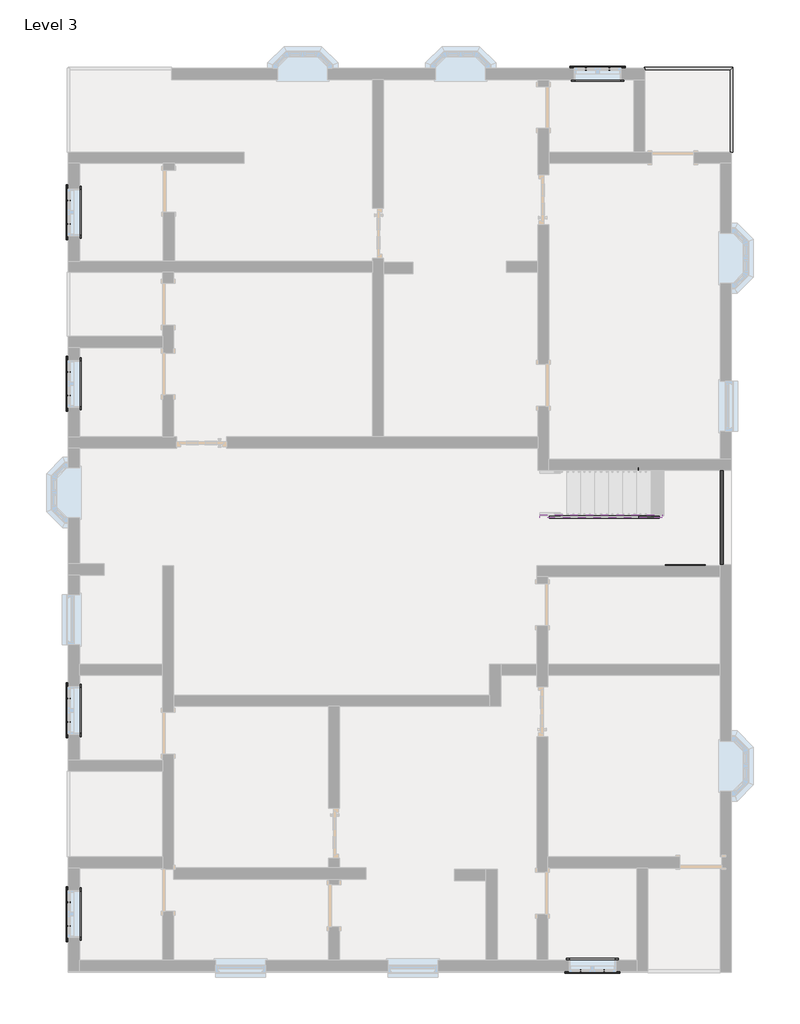
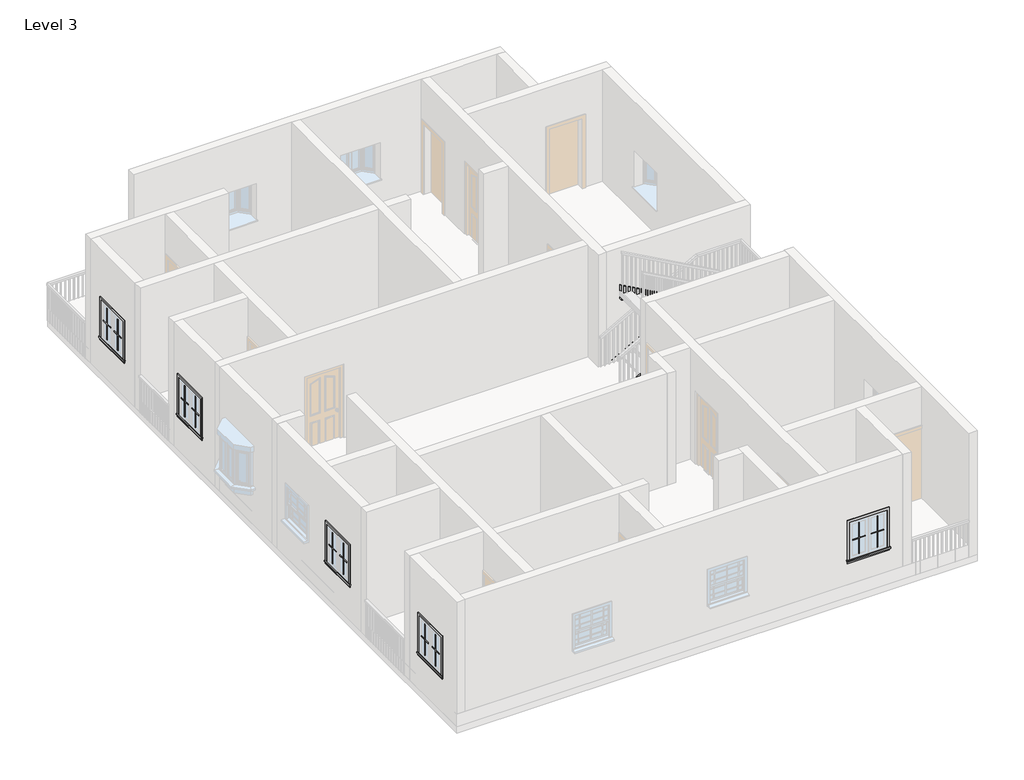
# One storey, part 4 of 4: 24 proxies, 5 members, 1 railing.
"""IFC4 building model written with IfcOpenShell, lengths in millimetres."""

from ifc_helpers import new_model, si_unit, frame, origin, place, context, project, spatial, polyline, outline, extrude, faceted_brep, transform, mapped, element, save
from components import muntin_pattern_2x2_muntin_pattern_2x2_b3fe6957, muntin_pattern_2x2_muntin_pattern_2x2_3e0ecaf2, trim_window_exterior_flat_with_sill_41619996, trim_window_interior_flat_picture_frame_51c85655

model = new_model("IFC4")

# Units and contexts
model_context = context("Model", 3, world=origin())
ifc_project = project(units=[si_unit("LENGTHUNIT", "METRE", prefix="MILLI")], contexts=[model_context])

# Site, building, storey
site = spatial("IfcSite", under=ifc_project)
building = spatial("IfcBuilding", under=site)
storey = spatial("IfcBuildingStorey", under=building, Name="Level 3", Elevation=6096.0)

# Proxies
placement = place(None, origin())
muntin_pattern_2x2_muntin_pattern_2x2_shape = muntin_pattern_2x2_muntin_pattern_2x2_b3fe6957(model_context)
element("IfcBuildingElementProxy", 1, Name="Muntin Pattern_2x2 : Muntin Pattern_2x2", ObjectType="Muntin Pattern_2x2 : Muntin Pattern_2x2", at=placement, inside=storey, context=model_context, shape_type="MappedRepresentation", body=[
    mapped(muntin_pattern_2x2_muntin_pattern_2x2_shape, transform((-7038.4808717, 5489.0318597, 7080.25), x_axis=(0.0, 1.0, 0.0), y_axis=(-1.0, 0.0, 0.0), z_axis=(0.0, 0.0, 1.0))),
])
element("IfcBuildingElementProxy", 2, Name="Muntin Pattern_2x2 : Muntin Pattern_2x2", ObjectType="Muntin Pattern_2x2 : Muntin Pattern_2x2", at=placement, inside=storey, context=model_context, shape_type="MappedRepresentation", body=[
    mapped(muntin_pattern_2x2_muntin_pattern_2x2_shape, transform((-7038.4808717, 2366.9422293, 7080.25), x_axis=(0.0, 1.0, 0.0), y_axis=(-1.0, 0.0, 0.0), z_axis=(0.0, 0.0, 1.0))),
])
element("IfcBuildingElementProxy", 3, Name="Muntin Pattern_2x2 : Muntin Pattern_2x2", ObjectType="Muntin Pattern_2x2 : Muntin Pattern_2x2", at=placement, inside=storey, context=model_context, shape_type="MappedRepresentation", body=[
    mapped(muntin_pattern_2x2_muntin_pattern_2x2_shape, transform((2376.9816283, 8312.1297293, 7080.25), x_axis=(1.0, 0.0, 0.0), y_axis=(0.0, 1.0, 0.0), z_axis=(0.0, 0.0, 1.0))),
])
element("IfcBuildingElementProxy", 4, Name="Muntin Pattern_2x2 : Muntin Pattern_2x2", ObjectType="Muntin Pattern_2x2 : Muntin Pattern_2x2", at=placement, inside=storey, context=model_context, shape_type="MappedRepresentation", body=[
    mapped(muntin_pattern_2x2_muntin_pattern_2x2_shape, transform((2710.3566283, -8102.6202707, 7080.25), x_axis=(-1.0, 0.0, 0.0), y_axis=(0.0, -1.0, 0.0), z_axis=(0.0, 0.0, 1.0))),
])
element("IfcBuildingElementProxy", 5, Name="Muntin Pattern_2x2 : Muntin Pattern_2x2", ObjectType="Muntin Pattern_2x2 : Muntin Pattern_2x2", at=placement, inside=storey, context=model_context, shape_type="MappedRepresentation", body=[
    mapped(muntin_pattern_2x2_muntin_pattern_2x2_shape, transform((-7038.4808717, -7285.0577707, 7080.25), x_axis=(0.0, 1.0, 0.0), y_axis=(-1.0, 0.0, 0.0), z_axis=(0.0, 0.0, 1.0))),
])
element("IfcBuildingElementProxy", 6, Name="Muntin Pattern_2x2 : Muntin Pattern_2x2", ObjectType="Muntin Pattern_2x2 : Muntin Pattern_2x2", at=placement, inside=storey, context=model_context, shape_type="MappedRepresentation", body=[
    mapped(muntin_pattern_2x2_muntin_pattern_2x2_shape, transform((-7038.4808717, -3576.6577707, 7080.25), x_axis=(0.0, 1.0, 0.0), y_axis=(-1.0, 0.0, 0.0), z_axis=(0.0, 0.0, 1.0))),
])
muntin_pattern_2x2_muntin_pattern_2x2_2_shape = muntin_pattern_2x2_muntin_pattern_2x2_3e0ecaf2(model_context)
element("IfcBuildingElementProxy", 7, Name="Muntin Pattern_2x2 : Muntin Pattern_2x2", ObjectType="Muntin Pattern_2x2 : Muntin Pattern_2x2", at=placement, inside=storey, context=model_context, shape_type="MappedRepresentation", body=[
    mapped(muntin_pattern_2x2_muntin_pattern_2x2_2_shape, transform((-7038.4808717, 5917.6568597, 7080.25), x_axis=(0.0, -1.0, 0.0), y_axis=(1.0, 0.0, 0.0), z_axis=(0.0, 0.0, 1.0))),
])
element("IfcBuildingElementProxy", 8, Name="Muntin Pattern_2x2 : Muntin Pattern_2x2", ObjectType="Muntin Pattern_2x2 : Muntin Pattern_2x2", at=placement, inside=storey, context=model_context, shape_type="MappedRepresentation", body=[
    mapped(muntin_pattern_2x2_muntin_pattern_2x2_2_shape, transform((-7038.4808717, 2795.5672293, 7080.25), x_axis=(0.0, -1.0, 0.0), y_axis=(1.0, 0.0, 0.0), z_axis=(0.0, 0.0, 1.0))),
])
element("IfcBuildingElementProxy", 9, Name="Muntin Pattern_2x2 : Muntin Pattern_2x2", ObjectType="Muntin Pattern_2x2 : Muntin Pattern_2x2", at=placement, inside=storey, context=model_context, shape_type="MappedRepresentation", body=[
    mapped(muntin_pattern_2x2_muntin_pattern_2x2_2_shape, transform((2805.6066283, 8312.1297293, 7080.25), x_axis=(-1.0, 0.0, 0.0), y_axis=(0.0, -1.0, 0.0), z_axis=(0.0, 0.0, 1.0))),
])
element("IfcBuildingElementProxy", 10, Name="Muntin Pattern_2x2 : Muntin Pattern_2x2", ObjectType="Muntin Pattern_2x2 : Muntin Pattern_2x2", at=placement, inside=storey, context=model_context, shape_type="MappedRepresentation", body=[
    mapped(muntin_pattern_2x2_muntin_pattern_2x2_2_shape, transform((2281.7316283, -8102.6202707, 7080.25), x_axis=(1.0, 0.0, 0.0), y_axis=(0.0, 1.0, 0.0), z_axis=(0.0, 0.0, 1.0))),
])
element("IfcBuildingElementProxy", 11, Name="Muntin Pattern_2x2 : Muntin Pattern_2x2", ObjectType="Muntin Pattern_2x2 : Muntin Pattern_2x2", at=placement, inside=storey, context=model_context, shape_type="MappedRepresentation", body=[
    mapped(muntin_pattern_2x2_muntin_pattern_2x2_2_shape, transform((-7038.4808717, -6856.4327707, 7080.25), x_axis=(0.0, -1.0, 0.0), y_axis=(1.0, 0.0, 0.0), z_axis=(0.0, 0.0, 1.0))),
])
element("IfcBuildingElementProxy", 12, Name="Muntin Pattern_2x2 : Muntin Pattern_2x2", ObjectType="Muntin Pattern_2x2 : Muntin Pattern_2x2", at=placement, inside=storey, context=model_context, shape_type="MappedRepresentation", body=[
    mapped(muntin_pattern_2x2_muntin_pattern_2x2_2_shape, transform((-7038.4808717, -3148.0327707, 7080.25), x_axis=(0.0, -1.0, 0.0), y_axis=(1.0, 0.0, 0.0), z_axis=(0.0, 0.0, 1.0))),
])
trim_window_exterior_flat_with_sill_shape = trim_window_exterior_flat_with_sill_41619996(model_context)
element("IfcBuildingElementProxy", 13, Name="Trim-Window-Exterior-Flat : with Sill", ObjectType="Trim-Window-Exterior-Flat : with Sill", at=placement, inside=storey, context=model_context, shape_type="MappedRepresentation", body=[
    mapped(trim_window_exterior_flat_with_sill_shape, transform((-7048.0058717, 5703.3443597, 7924.8), x_axis=(0.0, -1.0, 0.0), y_axis=(0.0, 0.0, 1.0), z_axis=(-1.0, 0.0, 0.0))),
])
element("IfcBuildingElementProxy", 14, Name="Trim-Window-Exterior-Flat : with Sill", ObjectType="Trim-Window-Exterior-Flat : with Sill", at=placement, inside=storey, context=model_context, shape_type="MappedRepresentation", body=[
    mapped(trim_window_exterior_flat_with_sill_shape, transform((-7048.0058717, 2581.2547293, 7924.8), x_axis=(0.0, -1.0, 0.0), y_axis=(0.0, 0.0, 1.0), z_axis=(-1.0, 0.0, 0.0))),
])
element("IfcBuildingElementProxy", 15, Name="Trim-Window-Exterior-Flat : with Sill", ObjectType="Trim-Window-Exterior-Flat : with Sill", at=placement, inside=storey, context=model_context, shape_type="MappedRepresentation", body=[
    mapped(trim_window_exterior_flat_with_sill_shape, transform((2591.2941283, 8321.6547293, 7924.8), x_axis=(-1.0, 0.0, 0.0), y_axis=(0.0, 0.0, 1.0), z_axis=(0.0, 1.0, 0.0))),
])
element("IfcBuildingElementProxy", 16, Name="Trim-Window-Exterior-Flat : with Sill", ObjectType="Trim-Window-Exterior-Flat : with Sill", at=placement, inside=storey, context=model_context, shape_type="MappedRepresentation", body=[
    mapped(trim_window_exterior_flat_with_sill_shape, transform((2496.0441283, -8112.1452707, 7924.8), x_axis=(1.0, 0.0, 0.0), y_axis=(0.0, 0.0, 1.0), z_axis=(0.0, -1.0, 0.0))),
])
element("IfcBuildingElementProxy", 17, Name="Trim-Window-Exterior-Flat : with Sill", ObjectType="Trim-Window-Exterior-Flat : with Sill", at=placement, inside=storey, context=model_context, shape_type="MappedRepresentation", body=[
    mapped(trim_window_exterior_flat_with_sill_shape, transform((-7048.0058717, -7070.7452707, 7924.8), x_axis=(0.0, -1.0, 0.0), y_axis=(0.0, 0.0, 1.0), z_axis=(-1.0, 0.0, 0.0))),
])
element("IfcBuildingElementProxy", 18, Name="Trim-Window-Exterior-Flat : with Sill", ObjectType="Trim-Window-Exterior-Flat : with Sill", at=placement, inside=storey, context=model_context, shape_type="MappedRepresentation", body=[
    mapped(trim_window_exterior_flat_with_sill_shape, transform((-7048.0058717, -3362.3452707, 7924.8), x_axis=(0.0, -1.0, 0.0), y_axis=(0.0, 0.0, 1.0), z_axis=(-1.0, 0.0, 0.0))),
])
trim_window_interior_flat_picture_frame_shape = trim_window_interior_flat_picture_frame_51c85655(model_context)
element("IfcBuildingElementProxy", 19, Name="Trim-Window-Interior-Flat : Picture Frame", ObjectType="Trim-Window-Interior-Flat : Picture Frame", at=placement, inside=storey, context=model_context, shape_type="MappedRepresentation", body=[
    mapped(trim_window_interior_flat_picture_frame_shape, transform((-6844.8058717, 5703.3443597, 7924.8), x_axis=(0.0, 1.0, 0.0), y_axis=(0.0, 0.0, 1.0), z_axis=(1.0, 0.0, 0.0))),
])
element("IfcBuildingElementProxy", 20, Name="Trim-Window-Interior-Flat : Picture Frame", ObjectType="Trim-Window-Interior-Flat : Picture Frame", at=placement, inside=storey, context=model_context, shape_type="MappedRepresentation", body=[
    mapped(trim_window_interior_flat_picture_frame_shape, transform((-6844.8058717, 2581.2547293, 7924.8), x_axis=(0.0, 1.0, 0.0), y_axis=(0.0, 0.0, 1.0), z_axis=(1.0, 0.0, 0.0))),
])
element("IfcBuildingElementProxy", 21, Name="Trim-Window-Interior-Flat : Picture Frame", ObjectType="Trim-Window-Interior-Flat : Picture Frame", at=placement, inside=storey, context=model_context, shape_type="MappedRepresentation", body=[
    mapped(trim_window_interior_flat_picture_frame_shape, transform((2591.2941283, 8118.4547293, 7924.8), x_axis=(1.0, 0.0, 0.0), y_axis=(0.0, 0.0, 1.0), z_axis=(0.0, -1.0, 0.0))),
])
element("IfcBuildingElementProxy", 22, Name="Trim-Window-Interior-Flat : Picture Frame", ObjectType="Trim-Window-Interior-Flat : Picture Frame", at=placement, inside=storey, context=model_context, shape_type="MappedRepresentation", body=[
    mapped(trim_window_interior_flat_picture_frame_shape, transform((2496.0441283, -7908.9452707, 7924.8), x_axis=(-1.0, 0.0, 0.0), y_axis=(0.0, 0.0, 1.0), z_axis=(0.0, 1.0, 0.0))),
])
element("IfcBuildingElementProxy", 23, Name="Trim-Window-Interior-Flat : Picture Frame", ObjectType="Trim-Window-Interior-Flat : Picture Frame", at=placement, inside=storey, context=model_context, shape_type="MappedRepresentation", body=[
    mapped(trim_window_interior_flat_picture_frame_shape, transform((-6844.8058717, -7070.7452707, 7924.8), x_axis=(0.0, 1.0, 0.0), y_axis=(0.0, 0.0, 1.0), z_axis=(1.0, 0.0, 0.0))),
])
element("IfcBuildingElementProxy", 24, Name="Trim-Window-Interior-Flat : Picture Frame", ObjectType="Trim-Window-Interior-Flat : Picture Frame", at=placement, inside=storey, context=model_context, shape_type="MappedRepresentation", body=[
    mapped(trim_window_interior_flat_picture_frame_shape, transform((-6844.8058717, -3362.3452707, 7924.8), x_axis=(0.0, 1.0, 0.0), y_axis=(0.0, 0.0, 1.0), z_axis=(1.0, 0.0, 0.0))),
])

# Members
element("IfcMember", 25, ObjectType="Stringer - 2\" Width", at=placement, inside=storey, context=model_context, shape_type="SweptSolid", body=[
    extrude(outline(polyline([(6306.6757607, 1537.1941283), (6096.0, 1537.1941283), (6096.0, 1786.1766781), (7543.8, 4407.1563102), (7543.8, 3776.7834593), (6306.6757607, 1537.1941283)])), frame((0.0, 1006.4547293, 0.0), z_axis=(0.0, 1.0, 0.0), x_axis=(0.0, 0.0, 1.0)), (0.0, 0.0, 1.0), 50.8),
])
element("IfcMember", 26, ObjectType="Stringer - 2\" Width", at=placement, inside=storey, context=model_context, shape_type="SweptSolid", body=[
    extrude(outline(polyline([(4826.4941283, 1057.2547293), (4877.2941283, 1057.2547293), (4877.2941283, -714.2964201), (4826.4941283, -714.2964201), (4826.4941283, 1057.2547293)])), frame((0.0, 0.0, 7239.0), z_axis=(0.0, 0.0, 1.0), x_axis=(1.0, 0.0, 0.0)), (0.0, 0.0, 1.0), 304.8),
])
element("IfcMember", 27, ObjectType="Stringer - 2\" Width", at=placement, inside=storey, context=model_context, shape_type="SweptSolid", body=[
    extrude(outline(polyline([(7239.0, 4555.0346706), (8906.0215532, 1537.1941283), (8557.8106009, 1537.1941283), (7239.0, 3924.6618197), (7239.0, 4555.0346706)])), frame((0.0, -765.0964201, 0.0), z_axis=(0.0, 1.0, 0.0), x_axis=(0.0, 0.0, 1.0)), (0.0, 0.0, 1.0), 50.8),
])
element("IfcMember", 28, ObjectType="Stringer - 2\" Width", at=placement, inside=storey, context=model_context, shape_type="SweptSolid", body=[
    extrude(outline(polyline([(6306.6757607, 1537.1941283), (6096.0, 1537.1941283), (6096.0, 1786.1766781), (7161.4963497, 3715.0648053), (7509.7073019, 3715.0648053), (6306.6757607, 1537.1941283)])), frame((0.0, 130.1547293, 0.0), z_axis=(0.0, 1.0, 0.0), x_axis=(0.0, 0.0, 1.0)), (0.0, 0.0, 1.0), 50.8),
])
element("IfcMember", 29, ObjectType="Stringer - 2\" Width", at=placement, inside=storey, context=model_context, shape_type="SweptSolid", body=[
    extrude(outline(polyline([(7326.7177047, 3765.8648053), (7674.928657, 3765.8648053), (8906.0215532, 1537.1941283), (8557.8106009, 1537.1941283), (7326.7177047, 3765.8648053)])), frame((0.0, 142.8547293, 0.0), z_axis=(0.0, 1.0, 0.0), x_axis=(0.0, 0.0, 1.0)), (0.0, 0.0, 1.0), 50.8),
])

# Railing
element("IfcRailing", 30, ObjectType="Handrail - Rectangular", at=placement, inside=storey, context=model_context, shape_type="SolidModel", body=[
    faceted_brep([(3442.1941283, 8347.0547293, 7010.4), (3442.1941283, 8347.0547293, 6959.6), (3442.1941283, 8296.2547293, 6959.6), (3442.1941283, 8296.2547293, 7010.4), (5055.0941283, 8347.0547293, 7010.4), (5055.0941283, 8347.0547293, 6959.6), (5004.2941283, 8296.2547293, 6959.6), (5004.2941283, 8296.2547293, 7010.4), (5055.0941283, 6797.6547293, 7010.4), (5004.2941283, 6797.6547293, 7010.4), (5004.2941283, 6797.6547293, 6959.6), (5055.0941283, 6797.6547293, 6959.6)], [[[0, 1, 2, 3]], [[1, 0, 4, 5]], [[2, 1, 5, 6]], [[3, 2, 6, 7]], [[0, 3, 7, 4]], [[8, 9, 10, 11]], [[5, 4, 8, 11]], [[6, 5, 11, 10]], [[7, 6, 10, 9]], [[4, 7, 9, 8]]]),
    extrude(outline(polyline([(5020.1691283, 6908.7797293), (5039.2191283, 6908.7797293), (5039.2191283, 6889.7297293), (5020.1691283, 6889.7297293), (5020.1691283, 6908.7797293)])), frame((0.0, 0.0, 6096.0), z_axis=(0.0, 0.0, 1.0), x_axis=(1.0, 0.0, 0.0)), (0.0, 0.0, 1.0), 863.6),
    extrude(outline(polyline([(5020.1691283, 7010.3797293), (5039.2191283, 7010.3797293), (5039.2191283, 6991.3297293), (5020.1691283, 6991.3297293), (5020.1691283, 7010.3797293)])), frame((0.0, 0.0, 6096.0), z_axis=(0.0, 0.0, 1.0), x_axis=(1.0, 0.0, 0.0)), (0.0, 0.0, 1.0), 863.6),
    extrude(outline(polyline([(5020.1691283, 7111.9797293), (5039.2191283, 7111.9797293), (5039.2191283, 7092.9297293), (5020.1691283, 7092.9297293), (5020.1691283, 7111.9797293)])), frame((0.0, 0.0, 6096.0), z_axis=(0.0, 0.0, 1.0), x_axis=(1.0, 0.0, 0.0)), (0.0, 0.0, 1.0), 863.6),
    extrude(outline(polyline([(5020.1691283, 7213.5797293), (5039.2191283, 7213.5797293), (5039.2191283, 7194.5297293), (5020.1691283, 7194.5297293), (5020.1691283, 7213.5797293)])), frame((0.0, 0.0, 6096.0), z_axis=(0.0, 0.0, 1.0), x_axis=(1.0, 0.0, 0.0)), (0.0, 0.0, 1.0), 863.6),
    extrude(outline(polyline([(5020.1691283, 7315.1797293), (5039.2191283, 7315.1797293), (5039.2191283, 7296.1297293), (5020.1691283, 7296.1297293), (5020.1691283, 7315.1797293)])), frame((0.0, 0.0, 6096.0), z_axis=(0.0, 0.0, 1.0), x_axis=(1.0, 0.0, 0.0)), (0.0, 0.0, 1.0), 863.6),
    extrude(outline(polyline([(5020.1691283, 7416.7797293), (5039.2191283, 7416.7797293), (5039.2191283, 7397.7297293), (5020.1691283, 7397.7297293), (5020.1691283, 7416.7797293)])), frame((0.0, 0.0, 6096.0), z_axis=(0.0, 0.0, 1.0), x_axis=(1.0, 0.0, 0.0)), (0.0, 0.0, 1.0), 863.6),
    extrude(outline(polyline([(5020.1691283, 7518.3797293), (5039.2191283, 7518.3797293), (5039.2191283, 7499.3297293), (5020.1691283, 7499.3297293), (5020.1691283, 7518.3797293)])), frame((0.0, 0.0, 6096.0), z_axis=(0.0, 0.0, 1.0), x_axis=(1.0, 0.0, 0.0)), (0.0, 0.0, 1.0), 863.6),
    extrude(outline(polyline([(5020.1691283, 7619.9797293), (5039.2191283, 7619.9797293), (5039.2191283, 7600.9297293), (5020.1691283, 7600.9297293), (5020.1691283, 7619.9797293)])), frame((0.0, 0.0, 6096.0), z_axis=(0.0, 0.0, 1.0), x_axis=(1.0, 0.0, 0.0)), (0.0, 0.0, 1.0), 863.6),
    extrude(outline(polyline([(5020.1691283, 7721.5797293), (5039.2191283, 7721.5797293), (5039.2191283, 7702.5297293), (5020.1691283, 7702.5297293), (5020.1691283, 7721.5797293)])), frame((0.0, 0.0, 6096.0), z_axis=(0.0, 0.0, 1.0), x_axis=(1.0, 0.0, 0.0)), (0.0, 0.0, 1.0), 863.6),
    extrude(outline(polyline([(5020.1691283, 7823.1797293), (5039.2191283, 7823.1797293), (5039.2191283, 7804.1297293), (5020.1691283, 7804.1297293), (5020.1691283, 7823.1797293)])), frame((0.0, 0.0, 6096.0), z_axis=(0.0, 0.0, 1.0), x_axis=(1.0, 0.0, 0.0)), (0.0, 0.0, 1.0), 863.6),
    extrude(outline(polyline([(5020.1691283, 7924.7797293), (5039.2191283, 7924.7797293), (5039.2191283, 7905.7297293), (5020.1691283, 7905.7297293), (5020.1691283, 7924.7797293)])), frame((0.0, 0.0, 6096.0), z_axis=(0.0, 0.0, 1.0), x_axis=(1.0, 0.0, 0.0)), (0.0, 0.0, 1.0), 863.6),
    extrude(outline(polyline([(5020.1691283, 8026.3797293), (5039.2191283, 8026.3797293), (5039.2191283, 8007.3297293), (5020.1691283, 8007.3297293), (5020.1691283, 8026.3797293)])), frame((0.0, 0.0, 6096.0), z_axis=(0.0, 0.0, 1.0), x_axis=(1.0, 0.0, 0.0)), (0.0, 0.0, 1.0), 863.6),
    extrude(outline(polyline([(5020.1691283, 8127.9797293), (5039.2191283, 8127.9797293), (5039.2191283, 8108.9297293), (5020.1691283, 8108.9297293), (5020.1691283, 8127.9797293)])), frame((0.0, 0.0, 6096.0), z_axis=(0.0, 0.0, 1.0), x_axis=(1.0, 0.0, 0.0)), (0.0, 0.0, 1.0), 863.6),
    extrude(outline(polyline([(5020.1691283, 8229.5797293), (5039.2191283, 8229.5797293), (5039.2191283, 8210.5297293), (5020.1691283, 8210.5297293), (5020.1691283, 8229.5797293)])), frame((0.0, 0.0, 6096.0), z_axis=(0.0, 0.0, 1.0), x_axis=(1.0, 0.0, 0.0)), (0.0, 0.0, 1.0), 863.6),
    extrude(outline(polyline([(4956.6691283, 8312.1297293), (4956.6691283, 8331.1797293), (4975.7191283, 8331.1797293), (4975.7191283, 8312.1297293), (4956.6691283, 8312.1297293)])), frame((0.0, 0.0, 6096.0), z_axis=(0.0, 0.0, 1.0), x_axis=(1.0, 0.0, 0.0)), (0.0, 0.0, 1.0), 863.6),
    extrude(outline(polyline([(4855.0691283, 8312.1297293), (4855.0691283, 8331.1797293), (4874.1191283, 8331.1797293), (4874.1191283, 8312.1297293), (4855.0691283, 8312.1297293)])), frame((0.0, 0.0, 6096.0), z_axis=(0.0, 0.0, 1.0), x_axis=(1.0, 0.0, 0.0)), (0.0, 0.0, 1.0), 863.6),
    extrude(outline(polyline([(4753.4691283, 8312.1297293), (4753.4691283, 8331.1797293), (4772.5191283, 8331.1797293), (4772.5191283, 8312.1297293), (4753.4691283, 8312.1297293)])), frame((0.0, 0.0, 6096.0), z_axis=(0.0, 0.0, 1.0), x_axis=(1.0, 0.0, 0.0)), (0.0, 0.0, 1.0), 863.6),
    extrude(outline(polyline([(4651.8691283, 8312.1297293), (4651.8691283, 8331.1797293), (4670.9191283, 8331.1797293), (4670.9191283, 8312.1297293), (4651.8691283, 8312.1297293)])), frame((0.0, 0.0, 6096.0), z_axis=(0.0, 0.0, 1.0), x_axis=(1.0, 0.0, 0.0)), (0.0, 0.0, 1.0), 863.6),
    extrude(outline(polyline([(4550.2691283, 8312.1297293), (4550.2691283, 8331.1797293), (4569.3191283, 8331.1797293), (4569.3191283, 8312.1297293), (4550.2691283, 8312.1297293)])), frame((0.0, 0.0, 6096.0), z_axis=(0.0, 0.0, 1.0), x_axis=(1.0, 0.0, 0.0)), (0.0, 0.0, 1.0), 863.6),
    extrude(outline(polyline([(4448.6691283, 8312.1297293), (4448.6691283, 8331.1797293), (4467.7191283, 8331.1797293), (4467.7191283, 8312.1297293), (4448.6691283, 8312.1297293)])), frame((0.0, 0.0, 6096.0), z_axis=(0.0, 0.0, 1.0), x_axis=(1.0, 0.0, 0.0)), (0.0, 0.0, 1.0), 863.6),
    extrude(outline(polyline([(4347.0691283, 8312.1297293), (4347.0691283, 8331.1797293), (4366.1191283, 8331.1797293), (4366.1191283, 8312.1297293), (4347.0691283, 8312.1297293)])), frame((0.0, 0.0, 6096.0), z_axis=(0.0, 0.0, 1.0), x_axis=(1.0, 0.0, 0.0)), (0.0, 0.0, 1.0), 863.6),
    extrude(outline(polyline([(4245.4691283, 8312.1297293), (4245.4691283, 8331.1797293), (4264.5191283, 8331.1797293), (4264.5191283, 8312.1297293), (4245.4691283, 8312.1297293)])), frame((0.0, 0.0, 6096.0), z_axis=(0.0, 0.0, 1.0), x_axis=(1.0, 0.0, 0.0)), (0.0, 0.0, 1.0), 863.6),
    extrude(outline(polyline([(4143.8691283, 8312.1297293), (4143.8691283, 8331.1797293), (4162.9191283, 8331.1797293), (4162.9191283, 8312.1297293), (4143.8691283, 8312.1297293)])), frame((0.0, 0.0, 6096.0), z_axis=(0.0, 0.0, 1.0), x_axis=(1.0, 0.0, 0.0)), (0.0, 0.0, 1.0), 863.6),
    extrude(outline(polyline([(4042.2691283, 8312.1297293), (4042.2691283, 8331.1797293), (4061.3191283, 8331.1797293), (4061.3191283, 8312.1297293), (4042.2691283, 8312.1297293)])), frame((0.0, 0.0, 6096.0), z_axis=(0.0, 0.0, 1.0), x_axis=(1.0, 0.0, 0.0)), (0.0, 0.0, 1.0), 863.6),
    extrude(outline(polyline([(3940.6691283, 8312.1297293), (3940.6691283, 8331.1797293), (3959.7191283, 8331.1797293), (3959.7191283, 8312.1297293), (3940.6691283, 8312.1297293)])), frame((0.0, 0.0, 6096.0), z_axis=(0.0, 0.0, 1.0), x_axis=(1.0, 0.0, 0.0)), (0.0, 0.0, 1.0), 863.6),
    extrude(outline(polyline([(3839.0691283, 8312.1297293), (3839.0691283, 8331.1797293), (3858.1191283, 8331.1797293), (3858.1191283, 8312.1297293), (3839.0691283, 8312.1297293)])), frame((0.0, 0.0, 6096.0), z_axis=(0.0, 0.0, 1.0), x_axis=(1.0, 0.0, 0.0)), (0.0, 0.0, 1.0), 863.6),
    extrude(outline(polyline([(3737.4691283, 8312.1297293), (3737.4691283, 8331.1797293), (3756.5191283, 8331.1797293), (3756.5191283, 8312.1297293), (3737.4691283, 8312.1297293)])), frame((0.0, 0.0, 6096.0), z_axis=(0.0, 0.0, 1.0), x_axis=(1.0, 0.0, 0.0)), (0.0, 0.0, 1.0), 863.6),
    extrude(outline(polyline([(3635.8691283, 8312.1297293), (3635.8691283, 8331.1797293), (3654.9191283, 8331.1797293), (3654.9191283, 8312.1297293), (3635.8691283, 8312.1297293)])), frame((0.0, 0.0, 6096.0), z_axis=(0.0, 0.0, 1.0), x_axis=(1.0, 0.0, 0.0)), (0.0, 0.0, 1.0), 863.6),
    extrude(outline(polyline([(3534.2691283, 8312.1297293), (3534.2691283, 8331.1797293), (3553.3191283, 8331.1797293), (3553.3191283, 8312.1297293), (3534.2691283, 8312.1297293)])), frame((0.0, 0.0, 6096.0), z_axis=(0.0, 0.0, 1.0), x_axis=(1.0, 0.0, 0.0)), (0.0, 0.0, 1.0), 863.6),
    extrude(outline(polyline([(5020.1691283, 8312.1297293), (5020.1691283, 8331.1797293), (5039.2191283, 8331.1797293), (5039.2191283, 8312.1297293), (5020.1691283, 8312.1297293)])), frame((0.0, 0.0, 6096.0), z_axis=(0.0, 0.0, 1.0), x_axis=(1.0, 0.0, 0.0)), (0.0, 0.0, 1.0), 863.6),
    extrude(outline(polyline([(5020.1691283, 6816.7047293), (5039.2191283, 6816.7047293), (5039.2191283, 6797.6547293), (5020.1691283, 6797.6547293), (5020.1691283, 6816.7047293)])), frame((0.0, 0.0, 6096.0), z_axis=(0.0, 0.0, 1.0), x_axis=(1.0, 0.0, 0.0)), (0.0, 0.0, 1.0), 863.6),
    extrude(outline(polyline([(3442.1941283, 8312.1297293), (3442.1941283, 8331.1797293), (3461.2441283, 8331.1797293), (3461.2441283, 8312.1297293), (3442.1941283, 8312.1297293)])), frame((0.0, 0.0, 6096.0), z_axis=(0.0, 0.0, 1.0), x_axis=(1.0, 0.0, 0.0)), (0.0, 0.0, 1.0), 863.6),
])

save(model, "model.ifc")

# Revit data of these elements
# Type "Muntin Pattern_2x2 : Muntin Pattern_2x2"
#   Width [instance default] = 4' - 0"
#   Thickness = 0' - 0 1/2"
#   Height [instance default] = 4' - 0"
#   Distance = 0' - 0 3/4"
#   Interior Material [instance default] = none
#   Exterior Material [instance default] = none
#   Default Elevation = 0
# Type "Trim-Window-Exterior-Flat : with Sill"
#   Trim Width = 0' - 2 1/4"
#   Trim Thickness_Picture Frame = 0' - 1 1/4"
#   Trim Thickness_with Sill = 0' - 0 3/4"
#   Sill Thickness = 0' - 1 1/4"
#   Opening Width [instance default] = 2' - 0"
#   Opening Height [instance default] = 3' - 0"
#   Default Elevation = 4' - 0"
#   Sill = yes
#   Picture Frame = no
#   Trim Material [instance default] = none
# Type "Trim-Window-Interior-Flat : Picture Frame"
#   Trim Thickness_Picture Frame = 0' - 1 1/4"
#   Trim Width = 0' - 2 1/4"
#   Trim Thickness_with Sill = 0' - 0 3/4"
#   Sill Thickness = 0' - 1 1/4"
#   Opening Width [instance default] = 2' - 0"
#   Opening Height [instance default] = 3' - 0"
#   Default Elevation = 4' - 0"
#   Sill = no
#   Picture Frame = yes
#   Trim Material [instance default] = none
# Type "Handrail - Rectangular"
#   Assembly Code = "C2010400"
#   built-in parameter 1008612 = 0.0416667 (stored number, unit not read)
#   built-in parameter 1008611 = 0.0416667 (stored number, unit not read)
#   built-in parameter 1008609 = 0.333333 (stored number, unit not read)
#   built-in parameter 1008604 = 0.166667 (stored number, unit not read)
#   built-in parameter 1008603 = 0.166667 (stored number, unit not read)
#   Railing Height = 3' - 0"
#   built-in parameter 1008630 = 2
#   built-in parameter 1008610 = 2
#   built-in parameter 1008618 = Baluster - Square : 3/4"
# Elements 1, 2, 3, 4, 5, 6, 7, 8, 9, 10, 11, 12 (IfcBuildingElementProxy, "Muntin Pattern_2x2 : Muntin Pattern_2x2")
#   Width = 0' - 11 5/8"
#   Height = 2' - 6 1/2"
#   Interior Material = Wood - Stained
#   Exterior Material = Clad - White
#   Phase Created = New Construction
#   Materials on its faces: "Clad - White", "Wood - Stained"
# Elements 13, 14, 15, 16, 17, 18 (IfcBuildingElementProxy, "Trim-Window-Exterior-Flat : with Sill")
#   Opening Width = 2' - 10"
#   Opening Height = 3' - 0"
#   Trim Material = Clad - White
#   Phase Created = New Construction
#   Materials on its faces: "Clad - White"
# Elements 19, 20, 21, 22, 23, 24 (IfcBuildingElementProxy, "Trim-Window-Interior-Flat : Picture Frame")
#   Opening Width = 2' - 10"
#   Opening Height = 3' - 0"
#   Trim Material = Wood - Stained
#   Phase Created = New Construction
#   Materials on its faces: "Wood - Stained"
# Elements 25, 27, 28, 29 (IfcMember, "Stringer - 2\" Width")
#   Phase Created = New Construction
# Element 26 (IfcMember, "Stringer - 2\" Width")
#   Phase Created = New Construction
#   Materials on its faces: "Render Material 41-165-0"
# Element 30 (IfcRailing, "Handrail - Rectangular")
#   Phase Created = New Construction
# Materials
#   "Clad - White": class "Wood", colour RGB 242 242 238, transparency 0, Cost = 0
#   "Wood - Stained": class "Wood", colour RGB 224 178 126, transparency 0, Cost = 0
#   "Render Material 41-165-0": colour RGB 41 165 0, transparency 0
